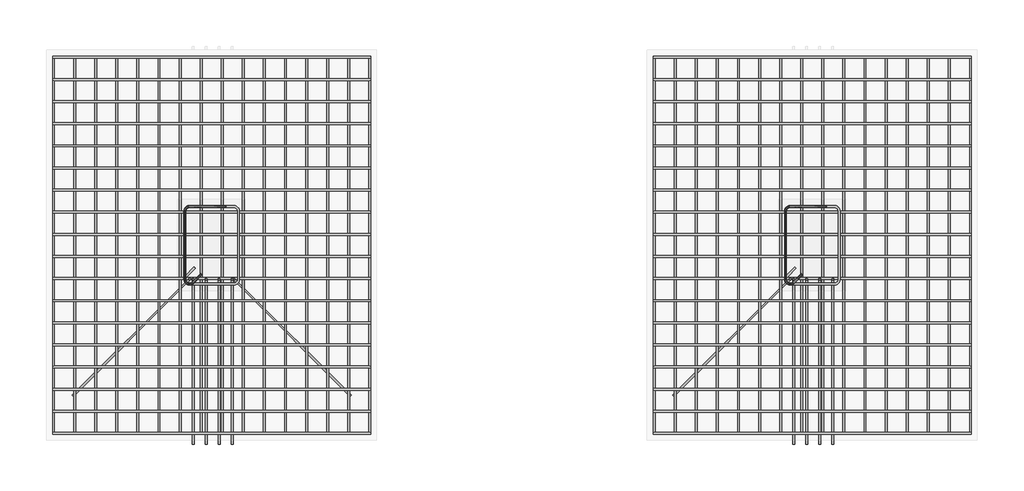
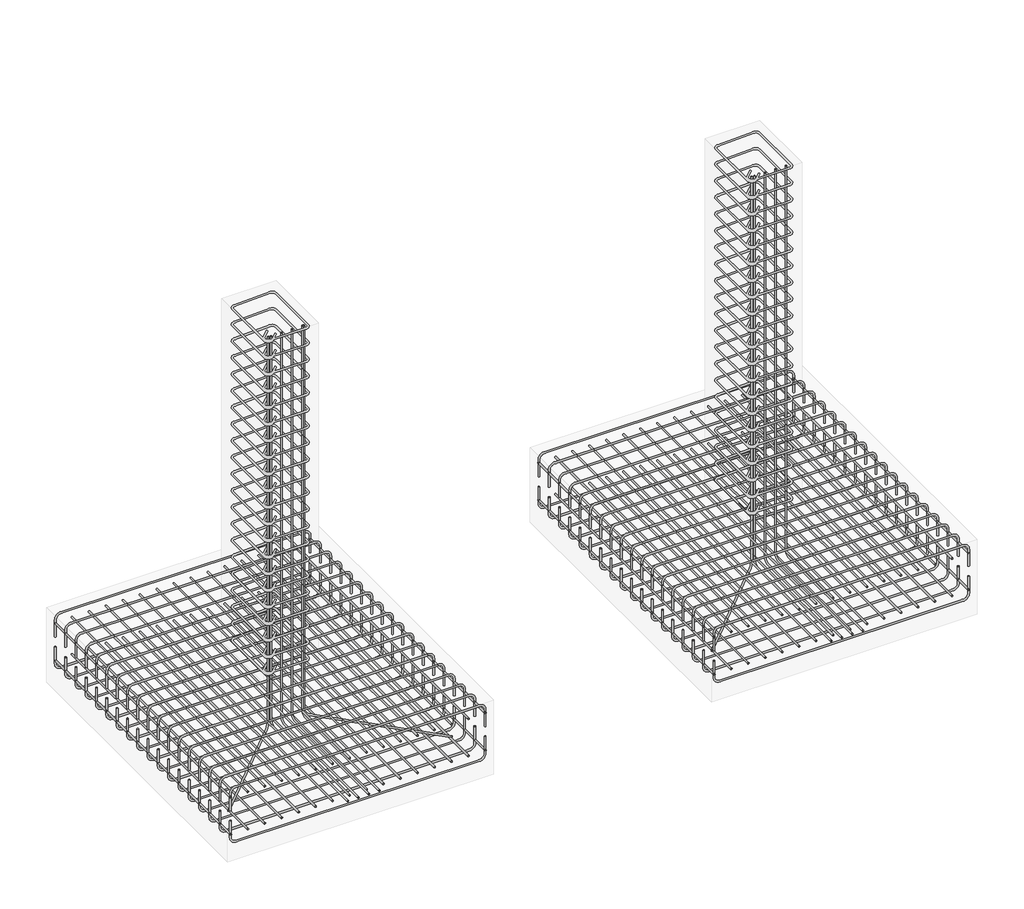
# One storey, part 3 of 33: 15 reinforcing bars.
"""IFC4 building model written with IfcOpenShell, lengths in millimetres."""

from ifc_helpers import new_model, si_unit, point, frame, origin, place, context, project, spatial, polyline, circle_curve, trimmed, segment, composite_curve, source, transform, mapped, element, save
from ifc_brep_helpers import swept_disk

model = new_model("IFC4")

# Units and contexts
model_context = context("Model", 3, world=origin())
ifc_project = project(units=[si_unit("LENGTHUNIT", "METRE", prefix="MILLI")], contexts=[model_context])

# Site, building, storey
site = spatial("IfcSite", under=ifc_project)
building = spatial("IfcBuilding", under=site)
storey = spatial("IfcBuildingStorey", under=building, Elevation=-3000.0)

# Reinforcing bars
placement = place(None, origin())
reinforcing_bar_shape = source(origin(), model_context, "Body", "SolidModel", [
    swept_disk(composite_curve([segment(polyline([(-10693.4642742, -7044.0608134, -3240.0), (-10693.4642742, -7044.0608134, -3092.7)]), True, "CONTINUOUS"), segment(trimmed(circle_curve(frame((-10647.1142742, -7044.0608134, -3092.7), z_axis=(0.0, 1.0, 0.0), x_axis=(-46.350000000000364, 0.0, 0.0)), 46.35), [point((-10693.4642742, -7044.0608134, -3092.7))], [point((-10647.1142742, -7044.0608134, -3046.35))], True, "CARTESIAN"), True, "CONTINUOUS"), segment(polyline([(-10647.1142742, -7044.0608134, -3046.35), (-8632.5142742, -7044.0608134, -3046.35)]), True, "CONTINUOUS"), segment(trimmed(circle_curve(frame((-8632.5142742, -7044.0608134, -3092.7), z_axis=(0.0, 1.0, 0.0), x_axis=(0.0, 0.0, 46.34999999999991)), 46.35), [point((-8632.5142742, -7044.0608134, -3046.35))], [point((-8586.1642742, -7044.0608134, -3092.7))], True, "CARTESIAN"), True, "CONTINUOUS"), segment(polyline([(-8586.1642742, -7044.0608134, -3092.7), (-8586.1642742, -7044.0608134, -3240.0)]), True, "CONTINUOUS")], self_intersect=False), 6.35),
])
element("IfcReinforcingBar", 1, at=placement, inside=storey, context=model_context, shape_type="MappedRepresentation", body=[
    mapped(reinforcing_bar_shape, transform((0.0, 0.0, 0.0), x_axis=(1.0, 0.0, 0.0), y_axis=(0.0, 1.0, 0.0), z_axis=(0.0, 0.0, 1.0))),
    mapped(reinforcing_bar_shape, transform((0.0, -147.4882353, 0.0), x_axis=(1.0, 0.0, 0.0), y_axis=(0.0, 1.0, 0.0), z_axis=(0.0, 0.0, 1.0))),
    mapped(reinforcing_bar_shape, transform((0.0, -294.9764706, 0.0), x_axis=(1.0, 0.0, 0.0), y_axis=(0.0, 1.0, 0.0), z_axis=(0.0, 0.0, 1.0))),
    mapped(reinforcing_bar_shape, transform((0.0, -442.4647059, 0.0), x_axis=(1.0, 0.0, 0.0), y_axis=(0.0, 1.0, 0.0), z_axis=(0.0, 0.0, 1.0))),
    mapped(reinforcing_bar_shape, transform((0.0, -589.9529412, 0.0), x_axis=(1.0, 0.0, 0.0), y_axis=(0.0, 1.0, 0.0), z_axis=(0.0, 0.0, 1.0))),
    mapped(reinforcing_bar_shape, transform((0.0, -737.4411765, 0.0), x_axis=(1.0, 0.0, 0.0), y_axis=(0.0, 1.0, 0.0), z_axis=(0.0, 0.0, 1.0))),
    mapped(reinforcing_bar_shape, transform((0.0, -884.9294118, 0.0), x_axis=(1.0, 0.0, 0.0), y_axis=(0.0, 1.0, 0.0), z_axis=(0.0, 0.0, 1.0))),
    mapped(reinforcing_bar_shape, transform((0.0, -1032.4176471, 0.0), x_axis=(1.0, 0.0, 0.0), y_axis=(0.0, 1.0, 0.0), z_axis=(0.0, 0.0, 1.0))),
    mapped(reinforcing_bar_shape, transform((0.0, -1179.9058824, 0.0), x_axis=(1.0, 0.0, 0.0), y_axis=(0.0, 1.0, 0.0), z_axis=(0.0, 0.0, 1.0))),
    mapped(reinforcing_bar_shape, transform((0.0, -1327.3941176, 0.0), x_axis=(1.0, 0.0, 0.0), y_axis=(0.0, 1.0, 0.0), z_axis=(0.0, 0.0, 1.0))),
    mapped(reinforcing_bar_shape, transform((0.0, -1474.8823529, 0.0), x_axis=(1.0, 0.0, 0.0), y_axis=(0.0, 1.0, 0.0), z_axis=(0.0, 0.0, 1.0))),
    mapped(reinforcing_bar_shape, transform((0.0, -1622.3705882, 0.0), x_axis=(1.0, 0.0, 0.0), y_axis=(0.0, 1.0, 0.0), z_axis=(0.0, 0.0, 1.0))),
    mapped(reinforcing_bar_shape, transform((0.0, -1769.8588235, 0.0), x_axis=(1.0, 0.0, 0.0), y_axis=(0.0, 1.0, 0.0), z_axis=(0.0, 0.0, 1.0))),
    mapped(reinforcing_bar_shape, transform((0.0, -1917.3470588, 0.0), x_axis=(1.0, 0.0, 0.0), y_axis=(0.0, 1.0, 0.0), z_axis=(0.0, 0.0, 1.0))),
    mapped(reinforcing_bar_shape, transform((0.0, -2064.8352941, 0.0), x_axis=(1.0, 0.0, 0.0), y_axis=(0.0, 1.0, 0.0), z_axis=(0.0, 0.0, 1.0))),
    mapped(reinforcing_bar_shape, transform((0.0, -2212.3235294, 0.0), x_axis=(1.0, 0.0, 0.0), y_axis=(0.0, 1.0, 0.0), z_axis=(0.0, 0.0, 1.0))),
    mapped(reinforcing_bar_shape, transform((0.0, -2359.8117647, 0.0), x_axis=(1.0, 0.0, 0.0), y_axis=(0.0, 1.0, 0.0), z_axis=(0.0, 0.0, 1.0))),
    mapped(reinforcing_bar_shape, transform((0.0, -2507.3, 0.0), x_axis=(1.0, 0.0, 0.0), y_axis=(0.0, 1.0, 0.0), z_axis=(0.0, 0.0, 1.0))),
])
reinforcing_bar_2_shape = source(origin(), model_context, "Body", "SolidModel", [
    swept_disk(composite_curve([segment(polyline([(-8586.1642742, -7044.0608134, -3330.080452), (-8586.1642742, -7044.0608134, -3477.380452)]), True, "CONTINUOUS"), segment(trimmed(circle_curve(frame((-8632.5142742, -7044.0608134, -3477.380452), z_axis=(0.0, 1.0, 0.0), x_axis=(46.350000000000364, 0.0, 0.0)), 46.35), [point((-8586.1642742, -7044.0608134, -3477.380452))], [point((-8632.5142742, -7044.0608134, -3523.730452))], True, "CARTESIAN"), True, "CONTINUOUS"), segment(polyline([(-8632.5142742, -7044.0608134, -3523.730452), (-10647.1142742, -7044.0608134, -3523.730452)]), True, "CONTINUOUS"), segment(trimmed(circle_curve(frame((-10647.1142742, -7044.0608134, -3477.380452), z_axis=(0.0, 1.0, 0.0), x_axis=(0.0, 0.0, -46.34999999999991)), 46.35), [point((-10647.1142742, -7044.0608134, -3523.730452))], [point((-10693.4642742, -7044.0608134, -3477.380452))], True, "CARTESIAN"), True, "CONTINUOUS"), segment(polyline([(-10693.4642742, -7044.0608134, -3477.380452), (-10693.4642742, -7044.0608134, -3330.080452)]), True, "CONTINUOUS")], self_intersect=False), 6.35),
])
element("IfcReinforcingBar", 2, at=placement, inside=storey, context=model_context, shape_type="MappedRepresentation", body=[
    mapped(reinforcing_bar_2_shape, transform((0.0, 0.0, 0.0), x_axis=(1.0, 0.0, 0.0), y_axis=(0.0, 1.0, 0.0), z_axis=(0.0, 0.0, 1.0))),
    mapped(reinforcing_bar_2_shape, transform((0.0, -147.4882353, 0.0), x_axis=(1.0, 0.0, 0.0), y_axis=(0.0, 1.0, 0.0), z_axis=(0.0, 0.0, 1.0))),
    mapped(reinforcing_bar_2_shape, transform((0.0, -294.9764706, 0.0), x_axis=(1.0, 0.0, 0.0), y_axis=(0.0, 1.0, 0.0), z_axis=(0.0, 0.0, 1.0))),
    mapped(reinforcing_bar_2_shape, transform((0.0, -442.4647059, 0.0), x_axis=(1.0, 0.0, 0.0), y_axis=(0.0, 1.0, 0.0), z_axis=(0.0, 0.0, 1.0))),
    mapped(reinforcing_bar_2_shape, transform((0.0, -589.9529412, 0.0), x_axis=(1.0, 0.0, 0.0), y_axis=(0.0, 1.0, 0.0), z_axis=(0.0, 0.0, 1.0))),
    mapped(reinforcing_bar_2_shape, transform((0.0, -737.4411765, 0.0), x_axis=(1.0, 0.0, 0.0), y_axis=(0.0, 1.0, 0.0), z_axis=(0.0, 0.0, 1.0))),
    mapped(reinforcing_bar_2_shape, transform((0.0, -884.9294118, 0.0), x_axis=(1.0, 0.0, 0.0), y_axis=(0.0, 1.0, 0.0), z_axis=(0.0, 0.0, 1.0))),
    mapped(reinforcing_bar_2_shape, transform((0.0, -1032.4176471, 0.0), x_axis=(1.0, 0.0, 0.0), y_axis=(0.0, 1.0, 0.0), z_axis=(0.0, 0.0, 1.0))),
    mapped(reinforcing_bar_2_shape, transform((0.0, -1179.9058824, 0.0), x_axis=(1.0, 0.0, 0.0), y_axis=(0.0, 1.0, 0.0), z_axis=(0.0, 0.0, 1.0))),
    mapped(reinforcing_bar_2_shape, transform((0.0, -1327.3941176, 0.0), x_axis=(1.0, 0.0, 0.0), y_axis=(0.0, 1.0, 0.0), z_axis=(0.0, 0.0, 1.0))),
    mapped(reinforcing_bar_2_shape, transform((0.0, -1474.8823529, 0.0), x_axis=(1.0, 0.0, 0.0), y_axis=(0.0, 1.0, 0.0), z_axis=(0.0, 0.0, 1.0))),
    mapped(reinforcing_bar_2_shape, transform((0.0, -1622.3705882, 0.0), x_axis=(1.0, 0.0, 0.0), y_axis=(0.0, 1.0, 0.0), z_axis=(0.0, 0.0, 1.0))),
    mapped(reinforcing_bar_2_shape, transform((0.0, -1769.8588235, 0.0), x_axis=(1.0, 0.0, 0.0), y_axis=(0.0, 1.0, 0.0), z_axis=(0.0, 0.0, 1.0))),
    mapped(reinforcing_bar_2_shape, transform((0.0, -1917.3470588, 0.0), x_axis=(1.0, 0.0, 0.0), y_axis=(0.0, 1.0, 0.0), z_axis=(0.0, 0.0, 1.0))),
    mapped(reinforcing_bar_2_shape, transform((0.0, -2064.8352941, 0.0), x_axis=(1.0, 0.0, 0.0), y_axis=(0.0, 1.0, 0.0), z_axis=(0.0, 0.0, 1.0))),
    mapped(reinforcing_bar_2_shape, transform((0.0, -2212.3235294, 0.0), x_axis=(1.0, 0.0, 0.0), y_axis=(0.0, 1.0, 0.0), z_axis=(0.0, 0.0, 1.0))),
    mapped(reinforcing_bar_2_shape, transform((0.0, -2359.8117647, 0.0), x_axis=(1.0, 0.0, 0.0), y_axis=(0.0, 1.0, 0.0), z_axis=(0.0, 0.0, 1.0))),
    mapped(reinforcing_bar_2_shape, transform((0.0, -2507.3, 0.0), x_axis=(1.0, 0.0, 0.0), y_axis=(0.0, 1.0, 0.0), z_axis=(0.0, 0.0, 1.0))),
])
reinforcing_bar_3_shape = source(origin(), model_context, "Body", "SolidModel", [
    swept_disk(composite_curve([segment(polyline([(-8586.1642742, -9557.7108134, -3447.8614173), (-8586.1642742, -7037.7108134, -3447.8614173)]), True, "CONTINUOUS")], self_intersect=False), 6.35),
])
element("IfcReinforcingBar", 3, at=placement, inside=storey, context=model_context, shape_type="MappedRepresentation", body=[
    mapped(reinforcing_bar_3_shape, transform((0.0, 0.0, 0.0), x_axis=(1.0, 0.0, 0.0), y_axis=(0.0, 1.0, 0.0), z_axis=(0.0, 0.0, 1.0))),
    mapped(reinforcing_bar_3_shape, transform((-140.4866667, 0.0, 0.0), x_axis=(1.0, 0.0, 0.0), y_axis=(0.0, 1.0, 0.0), z_axis=(0.0, 0.0, 1.0))),
    mapped(reinforcing_bar_3_shape, transform((-280.9733333, 0.0, 0.0), x_axis=(1.0, 0.0, 0.0), y_axis=(0.0, 1.0, 0.0), z_axis=(0.0, 0.0, 1.0))),
    mapped(reinforcing_bar_3_shape, transform((-421.46, 0.0, 0.0), x_axis=(1.0, 0.0, 0.0), y_axis=(0.0, 1.0, 0.0), z_axis=(0.0, 0.0, 1.0))),
    mapped(reinforcing_bar_3_shape, transform((-561.9466667, 0.0, 0.0), x_axis=(1.0, 0.0, 0.0), y_axis=(0.0, 1.0, 0.0), z_axis=(0.0, 0.0, 1.0))),
    mapped(reinforcing_bar_3_shape, transform((-702.4333333, 0.0, 0.0), x_axis=(1.0, 0.0, 0.0), y_axis=(0.0, 1.0, 0.0), z_axis=(0.0, 0.0, 1.0))),
    mapped(reinforcing_bar_3_shape, transform((-842.92, 0.0, 0.0), x_axis=(1.0, 0.0, 0.0), y_axis=(0.0, 1.0, 0.0), z_axis=(0.0, 0.0, 1.0))),
    mapped(reinforcing_bar_3_shape, transform((-983.4066667, 0.0, 0.0), x_axis=(1.0, 0.0, 0.0), y_axis=(0.0, 1.0, 0.0), z_axis=(0.0, 0.0, 1.0))),
    mapped(reinforcing_bar_3_shape, transform((-1123.8933333, 0.0, 0.0), x_axis=(1.0, 0.0, 0.0), y_axis=(0.0, 1.0, 0.0), z_axis=(0.0, 0.0, 1.0))),
    mapped(reinforcing_bar_3_shape, transform((-1264.38, 0.0, 0.0), x_axis=(1.0, 0.0, 0.0), y_axis=(0.0, 1.0, 0.0), z_axis=(0.0, 0.0, 1.0))),
    mapped(reinforcing_bar_3_shape, transform((-1404.8666667, 0.0, 0.0), x_axis=(1.0, 0.0, 0.0), y_axis=(0.0, 1.0, 0.0), z_axis=(0.0, 0.0, 1.0))),
    mapped(reinforcing_bar_3_shape, transform((-1545.3533333, 0.0, 0.0), x_axis=(1.0, 0.0, 0.0), y_axis=(0.0, 1.0, 0.0), z_axis=(0.0, 0.0, 1.0))),
    mapped(reinforcing_bar_3_shape, transform((-1685.84, 0.0, 0.0), x_axis=(1.0, 0.0, 0.0), y_axis=(0.0, 1.0, 0.0), z_axis=(0.0, 0.0, 1.0))),
    mapped(reinforcing_bar_3_shape, transform((-1826.3266667, 0.0, 0.0), x_axis=(1.0, 0.0, 0.0), y_axis=(0.0, 1.0, 0.0), z_axis=(0.0, 0.0, 1.0))),
    mapped(reinforcing_bar_3_shape, transform((-1966.8133333, 0.0, 0.0), x_axis=(1.0, 0.0, 0.0), y_axis=(0.0, 1.0, 0.0), z_axis=(0.0, 0.0, 1.0))),
    mapped(reinforcing_bar_3_shape, transform((-2107.3, 0.0, 0.0), x_axis=(1.0, 0.0, 0.0), y_axis=(0.0, 1.0, 0.0), z_axis=(0.0, 0.0, 1.0))),
])
reinforcing_bar_4_shape = source(origin(), model_context, "Body", "SolidModel", [
    swept_disk(composite_curve([segment(polyline([(-10693.4642742, -9557.7108134, -3122.7084113), (-10693.4642742, -7037.7108134, -3122.7084113)]), True, "CONTINUOUS")], self_intersect=False), 6.35),
])
element("IfcReinforcingBar", 4, at=placement, inside=storey, context=model_context, shape_type="MappedRepresentation", body=[
    mapped(reinforcing_bar_4_shape, transform((0.0, 0.0, 0.0), x_axis=(1.0, 0.0, 0.0), y_axis=(0.0, 1.0, 0.0), z_axis=(0.0, 0.0, 1.0))),
    mapped(reinforcing_bar_4_shape, transform((140.4866667, 0.0, 0.0), x_axis=(1.0, 0.0, 0.0), y_axis=(0.0, 1.0, 0.0), z_axis=(0.0, 0.0, 1.0))),
    mapped(reinforcing_bar_4_shape, transform((280.9733333, 0.0, 0.0), x_axis=(1.0, 0.0, 0.0), y_axis=(0.0, 1.0, 0.0), z_axis=(0.0, 0.0, 1.0))),
    mapped(reinforcing_bar_4_shape, transform((421.46, 0.0, 0.0), x_axis=(1.0, 0.0, 0.0), y_axis=(0.0, 1.0, 0.0), z_axis=(0.0, 0.0, 1.0))),
    mapped(reinforcing_bar_4_shape, transform((561.9466667, 0.0, 0.0), x_axis=(1.0, 0.0, 0.0), y_axis=(0.0, 1.0, 0.0), z_axis=(0.0, 0.0, 1.0))),
    mapped(reinforcing_bar_4_shape, transform((702.4333333, 0.0, 0.0), x_axis=(1.0, 0.0, 0.0), y_axis=(0.0, 1.0, 0.0), z_axis=(0.0, 0.0, 1.0))),
    mapped(reinforcing_bar_4_shape, transform((842.92, 0.0, 0.0), x_axis=(1.0, 0.0, 0.0), y_axis=(0.0, 1.0, 0.0), z_axis=(0.0, 0.0, 1.0))),
    mapped(reinforcing_bar_4_shape, transform((983.4066667, 0.0, 0.0), x_axis=(1.0, 0.0, 0.0), y_axis=(0.0, 1.0, 0.0), z_axis=(0.0, 0.0, 1.0))),
    mapped(reinforcing_bar_4_shape, transform((1123.8933333, 0.0, 0.0), x_axis=(1.0, 0.0, 0.0), y_axis=(0.0, 1.0, 0.0), z_axis=(0.0, 0.0, 1.0))),
    mapped(reinforcing_bar_4_shape, transform((1264.38, 0.0, 0.0), x_axis=(1.0, 0.0, 0.0), y_axis=(0.0, 1.0, 0.0), z_axis=(0.0, 0.0, 1.0))),
    mapped(reinforcing_bar_4_shape, transform((1404.8666667, 0.0, 0.0), x_axis=(1.0, 0.0, 0.0), y_axis=(0.0, 1.0, 0.0), z_axis=(0.0, 0.0, 1.0))),
    mapped(reinforcing_bar_4_shape, transform((1545.3533333, 0.0, 0.0), x_axis=(1.0, 0.0, 0.0), y_axis=(0.0, 1.0, 0.0), z_axis=(0.0, 0.0, 1.0))),
    mapped(reinforcing_bar_4_shape, transform((1685.84, 0.0, 0.0), x_axis=(1.0, 0.0, 0.0), y_axis=(0.0, 1.0, 0.0), z_axis=(0.0, 0.0, 1.0))),
    mapped(reinforcing_bar_4_shape, transform((1826.3266667, 0.0, 0.0), x_axis=(1.0, 0.0, 0.0), y_axis=(0.0, 1.0, 0.0), z_axis=(0.0, 0.0, 1.0))),
    mapped(reinforcing_bar_4_shape, transform((1966.8133333, 0.0, 0.0), x_axis=(1.0, 0.0, 0.0), y_axis=(0.0, 1.0, 0.0), z_axis=(0.0, 0.0, 1.0))),
    mapped(reinforcing_bar_4_shape, transform((2107.3, 0.0, 0.0), x_axis=(1.0, 0.0, 0.0), y_axis=(0.0, 1.0, 0.0), z_axis=(0.0, 0.0, 1.0))),
])
reinforcing_bar_5_shape = source(origin(), model_context, "Body", "SolidModel", [
    swept_disk(composite_curve([segment(polyline([(-14693.4642742, -7044.0608134, -3240.0), (-14693.4642742, -7044.0608134, -3092.7)]), True, "CONTINUOUS"), segment(trimmed(circle_curve(frame((-14647.1142742, -7044.0608134, -3092.7), z_axis=(0.0, 1.0, 0.0), x_axis=(-46.350000000000364, 0.0, 0.0)), 46.35), [point((-14693.4642742, -7044.0608134, -3092.7))], [point((-14647.1142742, -7044.0608134, -3046.35))], True, "CARTESIAN"), True, "CONTINUOUS"), segment(polyline([(-14647.1142742, -7044.0608134, -3046.35), (-12632.5142742, -7044.0608134, -3046.35)]), True, "CONTINUOUS"), segment(trimmed(circle_curve(frame((-12632.5142742, -7044.0608134, -3092.7), z_axis=(0.0, 1.0, 0.0), x_axis=(0.0, 0.0, 46.34999999999991)), 46.35), [point((-12632.5142742, -7044.0608134, -3046.35))], [point((-12586.1642742, -7044.0608134, -3092.7))], True, "CARTESIAN"), True, "CONTINUOUS"), segment(polyline([(-12586.1642742, -7044.0608134, -3092.7), (-12586.1642742, -7044.0608134, -3240.0)]), True, "CONTINUOUS")], self_intersect=False), 6.35),
])
element("IfcReinforcingBar", 5, at=placement, inside=storey, context=model_context, shape_type="MappedRepresentation", body=[
    mapped(reinforcing_bar_5_shape, transform((0.0, 0.0, 0.0), x_axis=(1.0, 0.0, 0.0), y_axis=(0.0, 1.0, 0.0), z_axis=(0.0, 0.0, 1.0))),
    mapped(reinforcing_bar_5_shape, transform((0.0, -147.4882353, 0.0), x_axis=(1.0, 0.0, 0.0), y_axis=(0.0, 1.0, 0.0), z_axis=(0.0, 0.0, 1.0))),
    mapped(reinforcing_bar_5_shape, transform((0.0, -294.9764706, 0.0), x_axis=(1.0, 0.0, 0.0), y_axis=(0.0, 1.0, 0.0), z_axis=(0.0, 0.0, 1.0))),
    mapped(reinforcing_bar_5_shape, transform((0.0, -442.4647059, 0.0), x_axis=(1.0, 0.0, 0.0), y_axis=(0.0, 1.0, 0.0), z_axis=(0.0, 0.0, 1.0))),
    mapped(reinforcing_bar_5_shape, transform((0.0, -589.9529412, 0.0), x_axis=(1.0, 0.0, 0.0), y_axis=(0.0, 1.0, 0.0), z_axis=(0.0, 0.0, 1.0))),
    mapped(reinforcing_bar_5_shape, transform((0.0, -737.4411765, 0.0), x_axis=(1.0, 0.0, 0.0), y_axis=(0.0, 1.0, 0.0), z_axis=(0.0, 0.0, 1.0))),
    mapped(reinforcing_bar_5_shape, transform((0.0, -884.9294118, 0.0), x_axis=(1.0, 0.0, 0.0), y_axis=(0.0, 1.0, 0.0), z_axis=(0.0, 0.0, 1.0))),
    mapped(reinforcing_bar_5_shape, transform((0.0, -1032.4176471, 0.0), x_axis=(1.0, 0.0, 0.0), y_axis=(0.0, 1.0, 0.0), z_axis=(0.0, 0.0, 1.0))),
    mapped(reinforcing_bar_5_shape, transform((0.0, -1179.9058824, 0.0), x_axis=(1.0, 0.0, 0.0), y_axis=(0.0, 1.0, 0.0), z_axis=(0.0, 0.0, 1.0))),
    mapped(reinforcing_bar_5_shape, transform((0.0, -1327.3941176, 0.0), x_axis=(1.0, 0.0, 0.0), y_axis=(0.0, 1.0, 0.0), z_axis=(0.0, 0.0, 1.0))),
    mapped(reinforcing_bar_5_shape, transform((0.0, -1474.8823529, 0.0), x_axis=(1.0, 0.0, 0.0), y_axis=(0.0, 1.0, 0.0), z_axis=(0.0, 0.0, 1.0))),
    mapped(reinforcing_bar_5_shape, transform((0.0, -1622.3705882, 0.0), x_axis=(1.0, 0.0, 0.0), y_axis=(0.0, 1.0, 0.0), z_axis=(0.0, 0.0, 1.0))),
    mapped(reinforcing_bar_5_shape, transform((0.0, -1769.8588235, 0.0), x_axis=(1.0, 0.0, 0.0), y_axis=(0.0, 1.0, 0.0), z_axis=(0.0, 0.0, 1.0))),
    mapped(reinforcing_bar_5_shape, transform((0.0, -1917.3470588, 0.0), x_axis=(1.0, 0.0, 0.0), y_axis=(0.0, 1.0, 0.0), z_axis=(0.0, 0.0, 1.0))),
    mapped(reinforcing_bar_5_shape, transform((0.0, -2064.8352941, 0.0), x_axis=(1.0, 0.0, 0.0), y_axis=(0.0, 1.0, 0.0), z_axis=(0.0, 0.0, 1.0))),
    mapped(reinforcing_bar_5_shape, transform((0.0, -2212.3235294, 0.0), x_axis=(1.0, 0.0, 0.0), y_axis=(0.0, 1.0, 0.0), z_axis=(0.0, 0.0, 1.0))),
    mapped(reinforcing_bar_5_shape, transform((0.0, -2359.8117647, 0.0), x_axis=(1.0, 0.0, 0.0), y_axis=(0.0, 1.0, 0.0), z_axis=(0.0, 0.0, 1.0))),
    mapped(reinforcing_bar_5_shape, transform((0.0, -2507.3, 0.0), x_axis=(1.0, 0.0, 0.0), y_axis=(0.0, 1.0, 0.0), z_axis=(0.0, 0.0, 1.0))),
])
reinforcing_bar_6_shape = source(origin(), model_context, "Body", "SolidModel", [
    swept_disk(composite_curve([segment(polyline([(-12586.1642742, -7044.0608134, -3330.080452), (-12586.1642742, -7044.0608134, -3477.380452)]), True, "CONTINUOUS"), segment(trimmed(circle_curve(frame((-12632.5142742, -7044.0608134, -3477.380452), z_axis=(0.0, 1.0, 0.0), x_axis=(46.350000000000364, 0.0, 0.0)), 46.35), [point((-12586.1642742, -7044.0608134, -3477.380452))], [point((-12632.5142742, -7044.0608134, -3523.730452))], True, "CARTESIAN"), True, "CONTINUOUS"), segment(polyline([(-12632.5142742, -7044.0608134, -3523.730452), (-14647.1142742, -7044.0608134, -3523.730452)]), True, "CONTINUOUS"), segment(trimmed(circle_curve(frame((-14647.1142742, -7044.0608134, -3477.380452), z_axis=(0.0, 1.0, 0.0), x_axis=(0.0, 0.0, -46.34999999999991)), 46.35), [point((-14647.1142742, -7044.0608134, -3523.730452))], [point((-14693.4642742, -7044.0608134, -3477.380452))], True, "CARTESIAN"), True, "CONTINUOUS"), segment(polyline([(-14693.4642742, -7044.0608134, -3477.380452), (-14693.4642742, -7044.0608134, -3330.080452)]), True, "CONTINUOUS")], self_intersect=False), 6.35),
])
element("IfcReinforcingBar", 6, at=placement, inside=storey, context=model_context, shape_type="MappedRepresentation", body=[
    mapped(reinforcing_bar_6_shape, transform((0.0, 0.0, 0.0), x_axis=(1.0, 0.0, 0.0), y_axis=(0.0, 1.0, 0.0), z_axis=(0.0, 0.0, 1.0))),
    mapped(reinforcing_bar_6_shape, transform((0.0, -147.4882353, 0.0), x_axis=(1.0, 0.0, 0.0), y_axis=(0.0, 1.0, 0.0), z_axis=(0.0, 0.0, 1.0))),
    mapped(reinforcing_bar_6_shape, transform((0.0, -294.9764706, 0.0), x_axis=(1.0, 0.0, 0.0), y_axis=(0.0, 1.0, 0.0), z_axis=(0.0, 0.0, 1.0))),
    mapped(reinforcing_bar_6_shape, transform((0.0, -442.4647059, 0.0), x_axis=(1.0, 0.0, 0.0), y_axis=(0.0, 1.0, 0.0), z_axis=(0.0, 0.0, 1.0))),
    mapped(reinforcing_bar_6_shape, transform((0.0, -589.9529412, 0.0), x_axis=(1.0, 0.0, 0.0), y_axis=(0.0, 1.0, 0.0), z_axis=(0.0, 0.0, 1.0))),
    mapped(reinforcing_bar_6_shape, transform((0.0, -737.4411765, 0.0), x_axis=(1.0, 0.0, 0.0), y_axis=(0.0, 1.0, 0.0), z_axis=(0.0, 0.0, 1.0))),
    mapped(reinforcing_bar_6_shape, transform((0.0, -884.9294118, 0.0), x_axis=(1.0, 0.0, 0.0), y_axis=(0.0, 1.0, 0.0), z_axis=(0.0, 0.0, 1.0))),
    mapped(reinforcing_bar_6_shape, transform((0.0, -1032.4176471, 0.0), x_axis=(1.0, 0.0, 0.0), y_axis=(0.0, 1.0, 0.0), z_axis=(0.0, 0.0, 1.0))),
    mapped(reinforcing_bar_6_shape, transform((0.0, -1179.9058824, 0.0), x_axis=(1.0, 0.0, 0.0), y_axis=(0.0, 1.0, 0.0), z_axis=(0.0, 0.0, 1.0))),
    mapped(reinforcing_bar_6_shape, transform((0.0, -1327.3941176, 0.0), x_axis=(1.0, 0.0, 0.0), y_axis=(0.0, 1.0, 0.0), z_axis=(0.0, 0.0, 1.0))),
    mapped(reinforcing_bar_6_shape, transform((0.0, -1474.8823529, 0.0), x_axis=(1.0, 0.0, 0.0), y_axis=(0.0, 1.0, 0.0), z_axis=(0.0, 0.0, 1.0))),
    mapped(reinforcing_bar_6_shape, transform((0.0, -1622.3705882, 0.0), x_axis=(1.0, 0.0, 0.0), y_axis=(0.0, 1.0, 0.0), z_axis=(0.0, 0.0, 1.0))),
    mapped(reinforcing_bar_6_shape, transform((0.0, -1769.8588235, 0.0), x_axis=(1.0, 0.0, 0.0), y_axis=(0.0, 1.0, 0.0), z_axis=(0.0, 0.0, 1.0))),
    mapped(reinforcing_bar_6_shape, transform((0.0, -1917.3470588, 0.0), x_axis=(1.0, 0.0, 0.0), y_axis=(0.0, 1.0, 0.0), z_axis=(0.0, 0.0, 1.0))),
    mapped(reinforcing_bar_6_shape, transform((0.0, -2064.8352941, 0.0), x_axis=(1.0, 0.0, 0.0), y_axis=(0.0, 1.0, 0.0), z_axis=(0.0, 0.0, 1.0))),
    mapped(reinforcing_bar_6_shape, transform((0.0, -2212.3235294, 0.0), x_axis=(1.0, 0.0, 0.0), y_axis=(0.0, 1.0, 0.0), z_axis=(0.0, 0.0, 1.0))),
    mapped(reinforcing_bar_6_shape, transform((0.0, -2359.8117647, 0.0), x_axis=(1.0, 0.0, 0.0), y_axis=(0.0, 1.0, 0.0), z_axis=(0.0, 0.0, 1.0))),
    mapped(reinforcing_bar_6_shape, transform((0.0, -2507.3, 0.0), x_axis=(1.0, 0.0, 0.0), y_axis=(0.0, 1.0, 0.0), z_axis=(0.0, 0.0, 1.0))),
])
reinforcing_bar_7_shape = source(origin(), model_context, "Body", "SolidModel", [
    swept_disk(composite_curve([segment(polyline([(-12586.1642742, -9557.7108134, -3447.8614173), (-12586.1642742, -7037.7108134, -3447.8614173)]), True, "CONTINUOUS")], self_intersect=False), 6.35),
])
element("IfcReinforcingBar", 7, at=placement, inside=storey, context=model_context, shape_type="MappedRepresentation", body=[
    mapped(reinforcing_bar_7_shape, transform((0.0, 0.0, 0.0), x_axis=(1.0, 0.0, 0.0), y_axis=(0.0, 1.0, 0.0), z_axis=(0.0, 0.0, 1.0))),
    mapped(reinforcing_bar_7_shape, transform((-140.4866667, 0.0, 0.0), x_axis=(1.0, 0.0, 0.0), y_axis=(0.0, 1.0, 0.0), z_axis=(0.0, 0.0, 1.0))),
    mapped(reinforcing_bar_7_shape, transform((-280.9733333, 0.0, 0.0), x_axis=(1.0, 0.0, 0.0), y_axis=(0.0, 1.0, 0.0), z_axis=(0.0, 0.0, 1.0))),
    mapped(reinforcing_bar_7_shape, transform((-421.46, 0.0, 0.0), x_axis=(1.0, 0.0, 0.0), y_axis=(0.0, 1.0, 0.0), z_axis=(0.0, 0.0, 1.0))),
    mapped(reinforcing_bar_7_shape, transform((-561.9466667, 0.0, 0.0), x_axis=(1.0, 0.0, 0.0), y_axis=(0.0, 1.0, 0.0), z_axis=(0.0, 0.0, 1.0))),
    mapped(reinforcing_bar_7_shape, transform((-702.4333333, 0.0, 0.0), x_axis=(1.0, 0.0, 0.0), y_axis=(0.0, 1.0, 0.0), z_axis=(0.0, 0.0, 1.0))),
    mapped(reinforcing_bar_7_shape, transform((-842.92, 0.0, 0.0), x_axis=(1.0, 0.0, 0.0), y_axis=(0.0, 1.0, 0.0), z_axis=(0.0, 0.0, 1.0))),
    mapped(reinforcing_bar_7_shape, transform((-983.4066667, 0.0, 0.0), x_axis=(1.0, 0.0, 0.0), y_axis=(0.0, 1.0, 0.0), z_axis=(0.0, 0.0, 1.0))),
    mapped(reinforcing_bar_7_shape, transform((-1123.8933333, 0.0, 0.0), x_axis=(1.0, 0.0, 0.0), y_axis=(0.0, 1.0, 0.0), z_axis=(0.0, 0.0, 1.0))),
    mapped(reinforcing_bar_7_shape, transform((-1264.38, 0.0, 0.0), x_axis=(1.0, 0.0, 0.0), y_axis=(0.0, 1.0, 0.0), z_axis=(0.0, 0.0, 1.0))),
    mapped(reinforcing_bar_7_shape, transform((-1404.8666667, 0.0, 0.0), x_axis=(1.0, 0.0, 0.0), y_axis=(0.0, 1.0, 0.0), z_axis=(0.0, 0.0, 1.0))),
    mapped(reinforcing_bar_7_shape, transform((-1545.3533333, 0.0, 0.0), x_axis=(1.0, 0.0, 0.0), y_axis=(0.0, 1.0, 0.0), z_axis=(0.0, 0.0, 1.0))),
    mapped(reinforcing_bar_7_shape, transform((-1685.84, 0.0, 0.0), x_axis=(1.0, 0.0, 0.0), y_axis=(0.0, 1.0, 0.0), z_axis=(0.0, 0.0, 1.0))),
    mapped(reinforcing_bar_7_shape, transform((-1826.3266667, 0.0, 0.0), x_axis=(1.0, 0.0, 0.0), y_axis=(0.0, 1.0, 0.0), z_axis=(0.0, 0.0, 1.0))),
    mapped(reinforcing_bar_7_shape, transform((-1966.8133333, 0.0, 0.0), x_axis=(1.0, 0.0, 0.0), y_axis=(0.0, 1.0, 0.0), z_axis=(0.0, 0.0, 1.0))),
    mapped(reinforcing_bar_7_shape, transform((-2107.3, 0.0, 0.0), x_axis=(1.0, 0.0, 0.0), y_axis=(0.0, 1.0, 0.0), z_axis=(0.0, 0.0, 1.0))),
])
reinforcing_bar_8_shape = source(origin(), model_context, "Body", "SolidModel", [
    swept_disk(composite_curve([segment(polyline([(-14693.4642742, -9557.7108134, -3122.7084113), (-14693.4642742, -7037.7108134, -3122.7084113)]), True, "CONTINUOUS")], self_intersect=False), 6.35),
])
element("IfcReinforcingBar", 8, at=placement, inside=storey, context=model_context, shape_type="MappedRepresentation", body=[
    mapped(reinforcing_bar_8_shape, transform((0.0, 0.0, 0.0), x_axis=(1.0, 0.0, 0.0), y_axis=(0.0, 1.0, 0.0), z_axis=(0.0, 0.0, 1.0))),
    mapped(reinforcing_bar_8_shape, transform((140.4866667, 0.0, 0.0), x_axis=(1.0, 0.0, 0.0), y_axis=(0.0, 1.0, 0.0), z_axis=(0.0, 0.0, 1.0))),
    mapped(reinforcing_bar_8_shape, transform((280.9733333, 0.0, 0.0), x_axis=(1.0, 0.0, 0.0), y_axis=(0.0, 1.0, 0.0), z_axis=(0.0, 0.0, 1.0))),
    mapped(reinforcing_bar_8_shape, transform((421.46, 0.0, 0.0), x_axis=(1.0, 0.0, 0.0), y_axis=(0.0, 1.0, 0.0), z_axis=(0.0, 0.0, 1.0))),
    mapped(reinforcing_bar_8_shape, transform((561.9466667, 0.0, 0.0), x_axis=(1.0, 0.0, 0.0), y_axis=(0.0, 1.0, 0.0), z_axis=(0.0, 0.0, 1.0))),
    mapped(reinforcing_bar_8_shape, transform((702.4333333, 0.0, 0.0), x_axis=(1.0, 0.0, 0.0), y_axis=(0.0, 1.0, 0.0), z_axis=(0.0, 0.0, 1.0))),
    mapped(reinforcing_bar_8_shape, transform((842.92, 0.0, 0.0), x_axis=(1.0, 0.0, 0.0), y_axis=(0.0, 1.0, 0.0), z_axis=(0.0, 0.0, 1.0))),
    mapped(reinforcing_bar_8_shape, transform((983.4066667, 0.0, 0.0), x_axis=(1.0, 0.0, 0.0), y_axis=(0.0, 1.0, 0.0), z_axis=(0.0, 0.0, 1.0))),
    mapped(reinforcing_bar_8_shape, transform((1123.8933333, 0.0, 0.0), x_axis=(1.0, 0.0, 0.0), y_axis=(0.0, 1.0, 0.0), z_axis=(0.0, 0.0, 1.0))),
    mapped(reinforcing_bar_8_shape, transform((1264.38, 0.0, 0.0), x_axis=(1.0, 0.0, 0.0), y_axis=(0.0, 1.0, 0.0), z_axis=(0.0, 0.0, 1.0))),
    mapped(reinforcing_bar_8_shape, transform((1404.8666667, 0.0, 0.0), x_axis=(1.0, 0.0, 0.0), y_axis=(0.0, 1.0, 0.0), z_axis=(0.0, 0.0, 1.0))),
    mapped(reinforcing_bar_8_shape, transform((1545.3533333, 0.0, 0.0), x_axis=(1.0, 0.0, 0.0), y_axis=(0.0, 1.0, 0.0), z_axis=(0.0, 0.0, 1.0))),
    mapped(reinforcing_bar_8_shape, transform((1685.84, 0.0, 0.0), x_axis=(1.0, 0.0, 0.0), y_axis=(0.0, 1.0, 0.0), z_axis=(0.0, 0.0, 1.0))),
    mapped(reinforcing_bar_8_shape, transform((1826.3266667, 0.0, 0.0), x_axis=(1.0, 0.0, 0.0), y_axis=(0.0, 1.0, 0.0), z_axis=(0.0, 0.0, 1.0))),
    mapped(reinforcing_bar_8_shape, transform((1966.8133333, 0.0, 0.0), x_axis=(1.0, 0.0, 0.0), y_axis=(0.0, 1.0, 0.0), z_axis=(0.0, 0.0, 1.0))),
    mapped(reinforcing_bar_8_shape, transform((2107.3, 0.0, 0.0), x_axis=(1.0, 0.0, 0.0), y_axis=(0.0, 1.0, 0.0), z_axis=(0.0, 0.0, 1.0))),
])
reinforcing_bar_9_shape = source(origin(), model_context, "Body", "SolidModel", [
    swept_disk(composite_curve([segment(polyline([(-13753.5385089, -8446.8994528, -2953.65), (-13809.2820718, -8502.6430158, -2953.65)]), True, "CONTINUOUS"), segment(trimmed(circle_curve(frame((-13787.1142742, -8524.8108134, -2953.65), z_axis=(0.0, 0.0, 1.0), x_axis=(-22.167797600000995, 22.167797599999176, 0.0)), 31.35), [point((-13809.2820718, -8502.6430158, -2953.65))], [point((-13787.1142742, -8556.1608134, -2953.65))], True, "CARTESIAN"), True, "CONTINUOUS"), segment(polyline([(-13787.1142742, -8556.1608134, -2953.65), (-13492.5142742, -8556.1608134, -2953.65)]), True, "CONTINUOUS"), segment(trimmed(circle_curve(frame((-13492.5142742, -8524.8108134, -2953.65), z_axis=(0.0, 0.0, 1.0), x_axis=(0.0, -31.350000000000364, 0.0)), 31.35), [point((-13492.5142742, -8556.1608134, -2953.65))], [point((-13461.1642742, -8524.8108134, -2953.65))], True, "CARTESIAN"), True, "CONTINUOUS"), segment(polyline([(-13461.1642742, -8524.8108134, -2953.65), (-13461.1642742, -8070.6108134, -2953.65)]), True, "CONTINUOUS"), segment(trimmed(circle_curve(frame((-13492.4944891, -8070.6108134, -2954.7636125), z_axis=(-0.0355219283344822, 0.0, 0.9993688971583016), x_axis=(31.33021489999919, 0.0, 1.1136124999998174)), 31.35), [point((-13461.1642742, -8070.6108134, -2953.65))], [point((-13492.4944891, -8039.2608134, -2954.7636125))], True, "CARTESIAN"), True, "CONTINUOUS"), segment(polyline([(-13492.4944891, -8039.2608134, -2954.7636125), (-13787.1340593, -8039.2608134, -2965.2363875)]), True, "CONTINUOUS"), segment(trimmed(circle_curve(frame((-13787.1340593, -8070.6108134, -2965.2363875), z_axis=(-0.0355219283344822, 0.0, 0.9993688971583016), x_axis=(0.0, 31.349999999999454, 0.0)), 31.35), [point((-13787.1340593, -8039.2608134, -2965.2363875))], [point((-13818.4642742, -8070.6108134, -2966.35))], True, "CARTESIAN"), True, "CONTINUOUS"), segment(polyline([(-13818.4642742, -8070.6108134, -2966.35), (-13818.4642742, -8524.8108134, -2966.35)]), True, "CONTINUOUS"), segment(trimmed(circle_curve(frame((-13787.1142742, -8524.8108134, -2966.35), z_axis=(0.0, 0.0, 1.0), x_axis=(-31.350000000000364, 0.0, 0.0)), 31.35), [point((-13818.4642742, -8524.8108134, -2966.35))], [point((-13764.9464766, -8546.978611, -2966.35))], True, "CARTESIAN"), True, "CONTINUOUS"), segment(polyline([(-13764.9464766, -8546.978611, -2966.35), (-13709.2029137, -8491.235048, -2966.35)]), True, "CONTINUOUS")], self_intersect=False), 6.35),
])
element("IfcReinforcingBar", 9, at=placement, inside=storey, context=model_context, shape_type="MappedRepresentation", body=[
    mapped(reinforcing_bar_9_shape, transform((0.0, 0.0, 0.0), x_axis=(1.0, 0.0, 0.0), y_axis=(0.0, 1.0, 0.0), z_axis=(0.0, 0.0, 1.0))),
    mapped(reinforcing_bar_9_shape, transform((0.0, 0.0, 145.365), x_axis=(1.0, 0.0, 0.0), y_axis=(0.0, 1.0, 0.0), z_axis=(0.0, 0.0, 1.0))),
    mapped(reinforcing_bar_9_shape, transform((0.0, 0.0, 290.73), x_axis=(1.0, 0.0, 0.0), y_axis=(0.0, 1.0, 0.0), z_axis=(0.0, 0.0, 1.0))),
    mapped(reinforcing_bar_9_shape, transform((0.0, 0.0, 436.095), x_axis=(1.0, 0.0, 0.0), y_axis=(0.0, 1.0, 0.0), z_axis=(0.0, 0.0, 1.0))),
    mapped(reinforcing_bar_9_shape, transform((0.0, 0.0, 581.46), x_axis=(1.0, 0.0, 0.0), y_axis=(0.0, 1.0, 0.0), z_axis=(0.0, 0.0, 1.0))),
    mapped(reinforcing_bar_9_shape, transform((0.0, 0.0, 726.825), x_axis=(1.0, 0.0, 0.0), y_axis=(0.0, 1.0, 0.0), z_axis=(0.0, 0.0, 1.0))),
    mapped(reinforcing_bar_9_shape, transform((0.0, 0.0, 872.19), x_axis=(1.0, 0.0, 0.0), y_axis=(0.0, 1.0, 0.0), z_axis=(0.0, 0.0, 1.0))),
    mapped(reinforcing_bar_9_shape, transform((0.0, 0.0, 1017.555), x_axis=(1.0, 0.0, 0.0), y_axis=(0.0, 1.0, 0.0), z_axis=(0.0, 0.0, 1.0))),
    mapped(reinforcing_bar_9_shape, transform((0.0, 0.0, 1162.92), x_axis=(1.0, 0.0, 0.0), y_axis=(0.0, 1.0, 0.0), z_axis=(0.0, 0.0, 1.0))),
    mapped(reinforcing_bar_9_shape, transform((0.0, 0.0, 1308.285), x_axis=(1.0, 0.0, 0.0), y_axis=(0.0, 1.0, 0.0), z_axis=(0.0, 0.0, 1.0))),
    mapped(reinforcing_bar_9_shape, transform((0.0, 0.0, 1453.65), x_axis=(1.0, 0.0, 0.0), y_axis=(0.0, 1.0, 0.0), z_axis=(0.0, 0.0, 1.0))),
    mapped(reinforcing_bar_9_shape, transform((0.0, 0.0, 1599.015), x_axis=(1.0, 0.0, 0.0), y_axis=(0.0, 1.0, 0.0), z_axis=(0.0, 0.0, 1.0))),
    mapped(reinforcing_bar_9_shape, transform((0.0, 0.0, 1744.38), x_axis=(1.0, 0.0, 0.0), y_axis=(0.0, 1.0, 0.0), z_axis=(0.0, 0.0, 1.0))),
    mapped(reinforcing_bar_9_shape, transform((0.0, 0.0, 1889.745), x_axis=(1.0, 0.0, 0.0), y_axis=(0.0, 1.0, 0.0), z_axis=(0.0, 0.0, 1.0))),
    mapped(reinforcing_bar_9_shape, transform((0.0, 0.0, 2035.11), x_axis=(1.0, 0.0, 0.0), y_axis=(0.0, 1.0, 0.0), z_axis=(0.0, 0.0, 1.0))),
    mapped(reinforcing_bar_9_shape, transform((0.0, 0.0, 2180.475), x_axis=(1.0, 0.0, 0.0), y_axis=(0.0, 1.0, 0.0), z_axis=(0.0, 0.0, 1.0))),
    mapped(reinforcing_bar_9_shape, transform((0.0, 0.0, 2325.84), x_axis=(1.0, 0.0, 0.0), y_axis=(0.0, 1.0, 0.0), z_axis=(0.0, 0.0, 1.0))),
    mapped(reinforcing_bar_9_shape, transform((0.0, 0.0, 2471.205), x_axis=(1.0, 0.0, 0.0), y_axis=(0.0, 1.0, 0.0), z_axis=(0.0, 0.0, 1.0))),
    mapped(reinforcing_bar_9_shape, transform((0.0, 0.0, 2616.57), x_axis=(1.0, 0.0, 0.0), y_axis=(0.0, 1.0, 0.0), z_axis=(0.0, 0.0, 1.0))),
    mapped(reinforcing_bar_9_shape, transform((0.0, 0.0, 2761.935), x_axis=(1.0, 0.0, 0.0), y_axis=(0.0, 1.0, 0.0), z_axis=(0.0, 0.0, 1.0))),
    mapped(reinforcing_bar_9_shape, transform((0.0, 0.0, 2907.3), x_axis=(1.0, 0.0, 0.0), y_axis=(0.0, 1.0, 0.0), z_axis=(0.0, 0.0, 1.0))),
])
element("IfcReinforcingBar", 10, at=placement, inside=storey, context=model_context, shape_type="SolidModel", body=[
    swept_disk(composite_curve([segment(polyline([(-13786.7956786, -8521.6339414, -40.0), (-13786.7956786, -8521.6339414, -3393.65)]), True, "CONTINUOUS"), segment(trimmed(circle_curve(frame((-13819.5700779, -8554.4083407, -3393.65), z_axis=(-0.7071067811865446, 0.7071067811865505, 0.0), x_axis=(32.77439930000037, 32.77439930000037, 0.0)), 46.35), [point((-13786.7956786, -8521.6339414, -3393.65))], [point((-13819.5700779, -8554.4083407, -3440.0))], True, "CARTESIAN"), True, "CONTINUOUS"), segment(polyline([(-13819.5700779, -8554.4083407, -3440.0), (-14564.6131379, -9299.4514007, -3440.0)]), True, "CONTINUOUS")], self_intersect=False), 6.35),
])
element("IfcReinforcingBar", 11, at=placement, inside=storey, context=model_context, shape_type="SolidModel", body=[
    swept_disk(composite_curve([segment(polyline([(-13492.8328699, -8521.6339414, -40.0), (-13492.8328699, -8521.6339414, -3393.65)]), True, "CONTINUOUS"), segment(trimmed(circle_curve(frame((-13460.0584706, -8554.4083407, -3393.65), z_axis=(-0.7071067811865493, -0.7071067811865459, 0.0), x_axis=(-32.77439929999855, 32.77439930000037, 0.0)), 46.35), [point((-13492.8328699, -8521.6339414, -3393.65))], [point((-13460.0584706, -8554.4083407, -3440.0))], True, "CARTESIAN"), True, "CONTINUOUS"), segment(polyline([(-13460.0584706, -8554.4083407, -3440.0), (-12715.0154106, -9299.4514007, -3440.0)]), True, "CONTINUOUS")], self_intersect=False), 6.35),
])
reinforcing_bar_10_shape = source(origin(), model_context, "Body", "SolidModel", [
    swept_disk(composite_curve([segment(polyline([(-13763.8841678, -8523.4938134, -40.0), (-13763.8841678, -8523.4938134, -3393.65)]), True, "CONTINUOUS"), segment(trimmed(circle_curve(frame((-13763.8841678, -8569.8438134, -3393.65), z_axis=(-1.0, 0.0, 0.0), x_axis=(0.0, 46.350000000000364, 0.0)), 46.35), [point((-13763.8841678, -8523.4938134, -3393.65))], [point((-13763.8841678, -8569.8438134, -3440.0))], True, "CARTESIAN"), True, "CONTINUOUS"), segment(polyline([(-13763.8841678, -8569.8438134, -3440.0), (-13763.8841678, -9623.4938134, -3440.0)]), True, "CONTINUOUS")], self_intersect=False), 6.35),
])
element("IfcReinforcingBar", 12, at=placement, inside=storey, context=model_context, shape_type="MappedRepresentation", body=[
    mapped(reinforcing_bar_10_shape, transform((0.0, 0.0, 0.0), x_axis=(1.0, 0.0, 0.0), y_axis=(0.0, 1.0, 0.0), z_axis=(0.0, 0.0, 1.0))),
    mapped(reinforcing_bar_10_shape, transform((86.8979716, 0.0, 0.0), x_axis=(1.0, 0.0, 0.0), y_axis=(0.0, 1.0, 0.0), z_axis=(0.0, 0.0, 1.0))),
    mapped(reinforcing_bar_10_shape, transform((173.7959432, 0.0, 0.0), x_axis=(1.0, 0.0, 0.0), y_axis=(0.0, 1.0, 0.0), z_axis=(0.0, 0.0, 1.0))),
    mapped(reinforcing_bar_10_shape, transform((260.6939148, 0.0, 0.0), x_axis=(1.0, 0.0, 0.0), y_axis=(0.0, 1.0, 0.0), z_axis=(0.0, 0.0, 1.0))),
])
reinforcing_bar_11_shape = source(origin(), model_context, "Body", "SolidModel", [
    swept_disk(composite_curve([segment(polyline([(-9753.5385089, -8446.8994528, -2953.65), (-9809.2820718, -8502.6430158, -2953.65)]), True, "CONTINUOUS"), segment(trimmed(circle_curve(frame((-9787.1142742, -8524.8108134, -2953.65), z_axis=(0.0, 0.0, 1.0), x_axis=(-22.167797600000995, 22.167797599999176, 0.0)), 31.35), [point((-9809.2820718, -8502.6430158, -2953.65))], [point((-9787.1142742, -8556.1608134, -2953.65))], True, "CARTESIAN"), True, "CONTINUOUS"), segment(polyline([(-9787.1142742, -8556.1608134, -2953.65), (-9492.5142742, -8556.1608134, -2953.65)]), True, "CONTINUOUS"), segment(trimmed(circle_curve(frame((-9492.5142742, -8524.8108134, -2953.65), z_axis=(0.0, 0.0, 1.0), x_axis=(0.0, -31.350000000000364, 0.0)), 31.35), [point((-9492.5142742, -8556.1608134, -2953.65))], [point((-9461.1642742, -8524.8108134, -2953.65))], True, "CARTESIAN"), True, "CONTINUOUS"), segment(polyline([(-9461.1642742, -8524.8108134, -2953.65), (-9461.1642742, -8070.6108134, -2953.65)]), True, "CONTINUOUS"), segment(trimmed(circle_curve(frame((-9492.4944891, -8070.6108134, -2954.7636125), z_axis=(-0.0355219283344822, 0.0, 0.9993688971583016), x_axis=(31.33021489999919, 0.0, 1.1136124999998174)), 31.35), [point((-9461.1642742, -8070.6108134, -2953.65))], [point((-9492.4944891, -8039.2608134, -2954.7636125))], True, "CARTESIAN"), True, "CONTINUOUS"), segment(polyline([(-9492.4944891, -8039.2608134, -2954.7636125), (-9787.1340593, -8039.2608134, -2965.2363875)]), True, "CONTINUOUS"), segment(trimmed(circle_curve(frame((-9787.1340593, -8070.6108134, -2965.2363875), z_axis=(-0.0355219283344822, 0.0, 0.9993688971583016), x_axis=(0.0, 31.349999999999454, 0.0)), 31.35), [point((-9787.1340593, -8039.2608134, -2965.2363875))], [point((-9818.4642742, -8070.6108134, -2966.35))], True, "CARTESIAN"), True, "CONTINUOUS"), segment(polyline([(-9818.4642742, -8070.6108134, -2966.35), (-9818.4642742, -8524.8108134, -2966.35)]), True, "CONTINUOUS"), segment(trimmed(circle_curve(frame((-9787.1142742, -8524.8108134, -2966.35), z_axis=(0.0, 0.0, 1.0), x_axis=(-31.350000000000364, 0.0, 0.0)), 31.35), [point((-9818.4642742, -8524.8108134, -2966.35))], [point((-9764.9464766, -8546.978611, -2966.35))], True, "CARTESIAN"), True, "CONTINUOUS"), segment(polyline([(-9764.9464766, -8546.978611, -2966.35), (-9709.2029137, -8491.235048, -2966.35)]), True, "CONTINUOUS")], self_intersect=False), 6.35),
])
element("IfcReinforcingBar", 13, at=placement, inside=storey, context=model_context, shape_type="MappedRepresentation", body=[
    mapped(reinforcing_bar_11_shape, transform((0.0, 0.0, 0.0), x_axis=(1.0, 0.0, 0.0), y_axis=(0.0, 1.0, 0.0), z_axis=(0.0, 0.0, 1.0))),
    mapped(reinforcing_bar_11_shape, transform((0.0, 0.0, 145.365), x_axis=(1.0, 0.0, 0.0), y_axis=(0.0, 1.0, 0.0), z_axis=(0.0, 0.0, 1.0))),
    mapped(reinforcing_bar_11_shape, transform((0.0, 0.0, 290.73), x_axis=(1.0, 0.0, 0.0), y_axis=(0.0, 1.0, 0.0), z_axis=(0.0, 0.0, 1.0))),
    mapped(reinforcing_bar_11_shape, transform((0.0, 0.0, 436.095), x_axis=(1.0, 0.0, 0.0), y_axis=(0.0, 1.0, 0.0), z_axis=(0.0, 0.0, 1.0))),
    mapped(reinforcing_bar_11_shape, transform((0.0, 0.0, 581.46), x_axis=(1.0, 0.0, 0.0), y_axis=(0.0, 1.0, 0.0), z_axis=(0.0, 0.0, 1.0))),
    mapped(reinforcing_bar_11_shape, transform((0.0, 0.0, 726.825), x_axis=(1.0, 0.0, 0.0), y_axis=(0.0, 1.0, 0.0), z_axis=(0.0, 0.0, 1.0))),
    mapped(reinforcing_bar_11_shape, transform((0.0, 0.0, 872.19), x_axis=(1.0, 0.0, 0.0), y_axis=(0.0, 1.0, 0.0), z_axis=(0.0, 0.0, 1.0))),
    mapped(reinforcing_bar_11_shape, transform((0.0, 0.0, 1017.555), x_axis=(1.0, 0.0, 0.0), y_axis=(0.0, 1.0, 0.0), z_axis=(0.0, 0.0, 1.0))),
    mapped(reinforcing_bar_11_shape, transform((0.0, 0.0, 1162.92), x_axis=(1.0, 0.0, 0.0), y_axis=(0.0, 1.0, 0.0), z_axis=(0.0, 0.0, 1.0))),
    mapped(reinforcing_bar_11_shape, transform((0.0, 0.0, 1308.285), x_axis=(1.0, 0.0, 0.0), y_axis=(0.0, 1.0, 0.0), z_axis=(0.0, 0.0, 1.0))),
    mapped(reinforcing_bar_11_shape, transform((0.0, 0.0, 1453.65), x_axis=(1.0, 0.0, 0.0), y_axis=(0.0, 1.0, 0.0), z_axis=(0.0, 0.0, 1.0))),
    mapped(reinforcing_bar_11_shape, transform((0.0, 0.0, 1599.015), x_axis=(1.0, 0.0, 0.0), y_axis=(0.0, 1.0, 0.0), z_axis=(0.0, 0.0, 1.0))),
    mapped(reinforcing_bar_11_shape, transform((0.0, 0.0, 1744.38), x_axis=(1.0, 0.0, 0.0), y_axis=(0.0, 1.0, 0.0), z_axis=(0.0, 0.0, 1.0))),
    mapped(reinforcing_bar_11_shape, transform((0.0, 0.0, 1889.745), x_axis=(1.0, 0.0, 0.0), y_axis=(0.0, 1.0, 0.0), z_axis=(0.0, 0.0, 1.0))),
    mapped(reinforcing_bar_11_shape, transform((0.0, 0.0, 2035.11), x_axis=(1.0, 0.0, 0.0), y_axis=(0.0, 1.0, 0.0), z_axis=(0.0, 0.0, 1.0))),
    mapped(reinforcing_bar_11_shape, transform((0.0, 0.0, 2180.475), x_axis=(1.0, 0.0, 0.0), y_axis=(0.0, 1.0, 0.0), z_axis=(0.0, 0.0, 1.0))),
    mapped(reinforcing_bar_11_shape, transform((0.0, 0.0, 2325.84), x_axis=(1.0, 0.0, 0.0), y_axis=(0.0, 1.0, 0.0), z_axis=(0.0, 0.0, 1.0))),
    mapped(reinforcing_bar_11_shape, transform((0.0, 0.0, 2471.205), x_axis=(1.0, 0.0, 0.0), y_axis=(0.0, 1.0, 0.0), z_axis=(0.0, 0.0, 1.0))),
    mapped(reinforcing_bar_11_shape, transform((0.0, 0.0, 2616.57), x_axis=(1.0, 0.0, 0.0), y_axis=(0.0, 1.0, 0.0), z_axis=(0.0, 0.0, 1.0))),
    mapped(reinforcing_bar_11_shape, transform((0.0, 0.0, 2761.935), x_axis=(1.0, 0.0, 0.0), y_axis=(0.0, 1.0, 0.0), z_axis=(0.0, 0.0, 1.0))),
    mapped(reinforcing_bar_11_shape, transform((0.0, 0.0, 2907.3), x_axis=(1.0, 0.0, 0.0), y_axis=(0.0, 1.0, 0.0), z_axis=(0.0, 0.0, 1.0))),
])
element("IfcReinforcingBar", 14, at=placement, inside=storey, context=model_context, shape_type="SolidModel", body=[
    swept_disk(composite_curve([segment(polyline([(-9786.7956786, -8521.6339414, -40.0), (-9786.7956786, -8521.6339414, -3393.65)]), True, "CONTINUOUS"), segment(trimmed(circle_curve(frame((-9819.5700779, -8554.4083407, -3393.65), z_axis=(-0.7071067811865446, 0.7071067811865505, 0.0), x_axis=(32.77439930000037, 32.77439930000037, 0.0)), 46.35), [point((-9786.7956786, -8521.6339414, -3393.65))], [point((-9819.5700779, -8554.4083407, -3440.0))], True, "CARTESIAN"), True, "CONTINUOUS"), segment(polyline([(-9819.5700779, -8554.4083407, -3440.0), (-10564.6131379, -9299.4514007, -3440.0)]), True, "CONTINUOUS")], self_intersect=False), 6.35),
])
reinforcing_bar_12_shape = source(origin(), model_context, "Body", "SolidModel", [
    swept_disk(composite_curve([segment(polyline([(-9763.8841678, -8523.4938134, -40.0), (-9763.8841678, -8523.4938134, -3393.65)]), True, "CONTINUOUS"), segment(trimmed(circle_curve(frame((-9763.8841678, -8569.8438134, -3393.65), z_axis=(-1.0, 0.0, 0.0), x_axis=(0.0, 46.350000000000364, 0.0)), 46.35), [point((-9763.8841678, -8523.4938134, -3393.65))], [point((-9763.8841678, -8569.8438134, -3440.0))], True, "CARTESIAN"), True, "CONTINUOUS"), segment(polyline([(-9763.8841678, -8569.8438134, -3440.0), (-9763.8841678, -9623.4938134, -3440.0)]), True, "CONTINUOUS")], self_intersect=False), 6.35),
])
element("IfcReinforcingBar", 15, at=placement, inside=storey, context=model_context, shape_type="MappedRepresentation", body=[
    mapped(reinforcing_bar_12_shape, transform((0.0, 0.0, 0.0), x_axis=(1.0, 0.0, 0.0), y_axis=(0.0, 1.0, 0.0), z_axis=(0.0, 0.0, 1.0))),
    mapped(reinforcing_bar_12_shape, transform((86.8979716, 0.0, 0.0), x_axis=(1.0, 0.0, 0.0), y_axis=(0.0, 1.0, 0.0), z_axis=(0.0, 0.0, 1.0))),
    mapped(reinforcing_bar_12_shape, transform((173.7959432, 0.0, 0.0), x_axis=(1.0, 0.0, 0.0), y_axis=(0.0, 1.0, 0.0), z_axis=(0.0, 0.0, 1.0))),
    mapped(reinforcing_bar_12_shape, transform((260.6939148, 0.0, 0.0), x_axis=(1.0, 0.0, 0.0), y_axis=(0.0, 1.0, 0.0), z_axis=(0.0, 0.0, 1.0))),
])

save(model, "model.ifc")

# Revit data of these elements
# Elements 1, 2, 3, 4, 5, 6, 7, 8, 9, 10, 11, 12, 13, 14, 15 (IfcReinforcingBar)
#   Phase Created = New Construction
